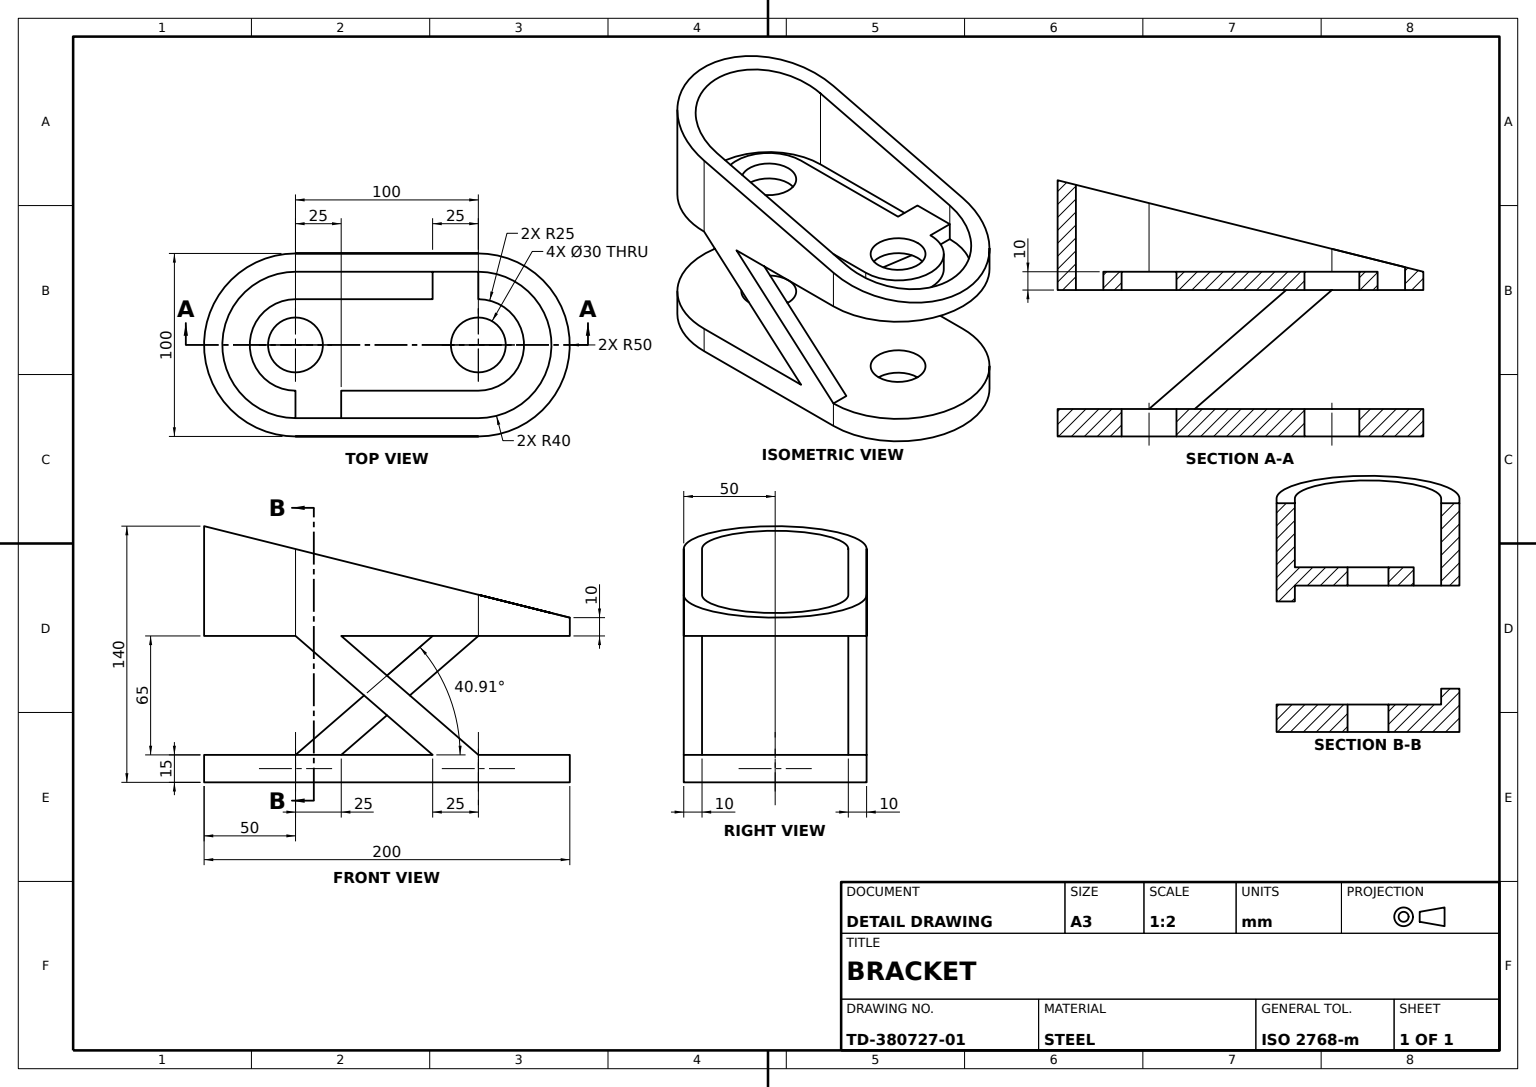
from build123d import *

# Parameters (mm, degrees)
LINK_PROFILES_SKETCH_R   = 15
BASE_LINK_PLATE_DEPTH    = 15
UPPER_START              = 90
UPPER_LINK_PLATE_DEPTH   = 10
LINK_START               = 15
LINK_SLOT_CUT_DEPTH      = 90
SLOT_START               = 80
SKETCH1_7_R              = 15
SLOT_TAB_BOSS_DEPTH      = 10
BRACE_STRUT_A_DEPTH      = 10
BRACE_WEB_A_SKETCH_W     = 25
BRACE_WEB_A_SKETCH_H     = 25
BRACE_WEB_A_DEPTH        = 10
BRACE_STRUT_B_DEPTH      = 10
BRACE_WEB_B_SKETCH_W     = 25
BRACE_WEB_B_SKETCH_H     = 25
BRACE_WEB_B_DEPTH        = 10
SLOTTED_START            = 90
SLOTTED_UPPER_WALL_DEPTH = 50
SIDE_TRIM_CUT_DEPTH      = 150


with BuildPart() as part:
    # Link Profiles Sketch → Base Link Plate (new body)
    with BuildSketch(Plane(origin=(0, 0, 0), x_dir=(1, 0, 0), z_dir=(0, 1, 0))):
        with BuildLine():
            Line((0, 50), (100, 50))
            ThreePointArc((100, 50), (150, 0), (100, -50))
            Line((100, -50), (0, -50))
            ThreePointArc((0, -50), (-50, 0), (0, 50))
        make_face()
        with Locations(Location((0, 0, 0), (0, 0, 270))):
            Circle(LINK_PROFILES_SKETCH_R, mode=Mode.SUBTRACT)
        with Locations(Location((100, 0, 0), (0, 0, 270))):
            Circle(LINK_PROFILES_SKETCH_R, mode=Mode.SUBTRACT)
    extrude(amount=BASE_LINK_PLATE_DEPTH)



with BuildPart() as body_2:
    # Sketch1_5 → Upper Link Plate (new body)
    with BuildSketch(Plane(origin=(0, 0, 0), x_dir=(1, 0, 0), z_dir=(0, 1, 0)).offset(UPPER_START)):
        with BuildLine():
            Line((0, 50), (100, 50))
            ThreePointArc((100, 50), (150, 0), (100, -50))
            Line((100, -50), (0, -50))
            ThreePointArc((0, -50), (-50, 0), (0, 50))
        make_face()
    extrude(amount=-UPPER_LINK_PLATE_DEPTH)

    # Sketch1_6 → Link Slot Cut (cut)
    with BuildSketch(Plane(origin=(0, 0, 0), x_dir=(1, 0, 0), z_dir=(0, 1, 0)).offset(LINK_START)):
        with BuildLine():
            Line((0, 40), (100, 40))
            ThreePointArc((100, 40), (140, 0), (100, -40))
            Line((100, -40), (0, -40))
            ThreePointArc((0, -40), (-40, 0), (0, 40))
        make_face()
    extrude(amount=LINK_SLOT_CUT_DEPTH, mode=Mode.SUBTRACT)


with BuildPart() as body_3:
    # Sketch1_7 → Slot Tab Boss (new body)
    with BuildSketch(Plane(origin=(0, 0, 0), x_dir=(1, 0, 0), z_dir=(0, 1, 0)).offset(SLOT_START)):
        with BuildLine():
            Line((0, 25), (100, 25))
            ThreePointArc((100, 25), (125, 0), (100, -25))
            Line((100, -25), (0, -25))
            ThreePointArc((0, -25), (-25, 0), (0, 25))
        make_face()
        with Locations(Location((0, 0, 0), (0, 0, 270))):
            Circle(SKETCH1_7_R, mode=Mode.SUBTRACT)
        with Locations(Location((100, 0, 0), (0, 0, 270))):
            Circle(SKETCH1_7_R, mode=Mode.SUBTRACT)
    extrude(amount=SLOT_TAB_BOSS_DEPTH)


with BuildPart() as part_1:
    add(part.part)

    add(body_2.part)  # Brace Strut A merges body 2
    # Brace Strut A Sketch → Brace Strut A (add)
    with BuildSketch(Plane.XY.offset(50)):
        Polygon((100, 0), (75, 0), (75, 15), (0, 80), (0, 90), (25, 90), (25, 80), (100, 15), align=None)
    extrude(amount=-BRACE_STRUT_A_DEPTH)


    add(body_3.part)  # Brace Web A merges body 3
    # Brace Web A Sketch → Brace Web A (add)
    with BuildSketch(Plane(origin=(0, 90, 0), x_dir=(1, 0, 0), z_dir=(0, 1, 0))):
        with Locations((12.5, -37.5)):
            Rectangle(BRACE_WEB_A_SKETCH_W, BRACE_WEB_A_SKETCH_H)
    extrude(amount=-BRACE_WEB_A_DEPTH)

    # Brace Strut B Sketch → Brace Strut B (add)
    with BuildSketch(Plane(origin=(0, 0, -50), x_dir=(-1, 0, 0), z_dir=(0, 0, -1))):
        Polygon((0, 0), (-25, 0), (-25, 15), (-100, 80), (-100, 90), (-75, 90), (-75, 80), (0, 15), align=None)
    extrude(amount=-BRACE_STRUT_B_DEPTH)

    # Brace Web B Sketch → Brace Web B (add)
    with BuildSketch(Plane(origin=(0, 90, 0), x_dir=(1, 0, 0), z_dir=(0, 1, 0))):
        with Locations((87.5, 37.5)):
            Rectangle(BRACE_WEB_B_SKETCH_W, BRACE_WEB_B_SKETCH_H)
    extrude(amount=-BRACE_WEB_B_DEPTH)

    # Sketch1_9 → Slotted Upper Wall (add)
    with BuildSketch(Plane(origin=(0, 0, 0), x_dir=(1, 0, 0), z_dir=(0, 1, 0)).offset(SLOTTED_START)):
        with BuildLine():
            Line((0, 50), (100, 50))
            ThreePointArc((100, 50), (150, 0), (100, -50))
            Line((100, -50), (0, -50))
            ThreePointArc((0, -50), (-50, 0), (0, 50))
        make_face()
        with BuildLine():
            Line((0, 40), (100, 40))
            ThreePointArc((100, 40), (140, 0), (100, -40))
            Line((100, -40), (0, -40))
            ThreePointArc((0, -40), (-40, 0), (0, 40))
        make_face(mode=Mode.SUBTRACT)
    extrude(amount=SLOTTED_UPPER_WALL_DEPTH)

    # Side Trim Sketch → Side Trim Cut (cut)
    with BuildSketch(Plane.XY.offset(50)):
        Polygon((150, 90), (-50, 140), (150, 140), align=None)
    extrude(amount=-SIDE_TRIM_CUT_DEPTH, mode=Mode.SUBTRACT)


solid = part_1.part
